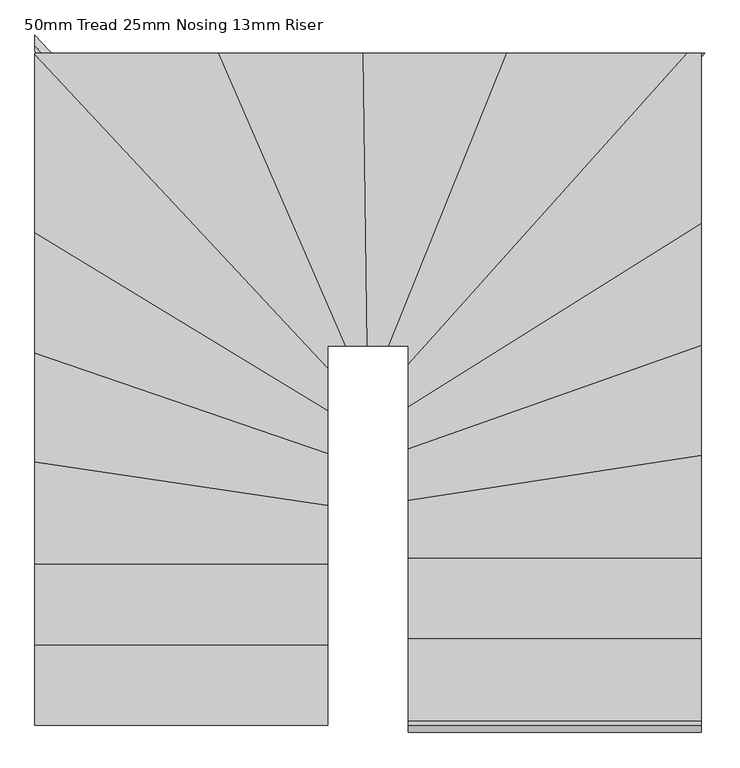
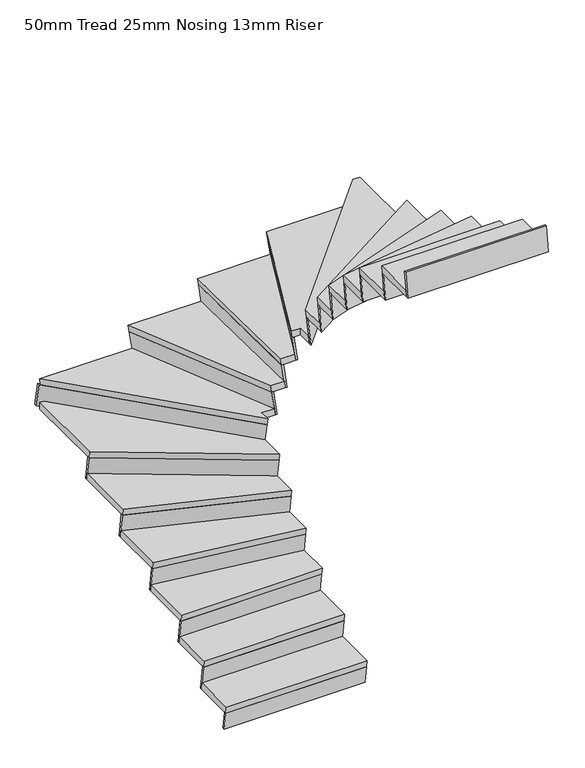
"""IFC4 building model written with IfcOpenShell, lengths in millimetres: stair flight geometry, 50mm Tread 25mm Nosing 13mm Riser."""

from ifc_helpers import new_model, si_unit, origin, place, context, project, spatial, faceted_brep, source, transform, mapped, element, save


def stair_flight_50mm_tread_25mm_nosing_13mm_riser_190ae62b(model_context):
    return source(origin(), model_context, "Body", "Brep", [
        faceted_brep([(10289.7497541, -1105.5848061, 179.2941176), (10289.7497541, -1098.6130213, 129.2941176), (9289.7239729, -1098.6130213, 129.2941176), (9289.7239729, -1105.5848061, 179.2941176), (9289.7239729, -1405.5848061, 179.2941176), (10289.7497541, -1405.5848061, 179.2941176), (10289.7497541, -1398.6130213, 129.2941176), (9289.7239729, -1398.6130213, 129.2941176)], [[[0, 1, 2, 3]], [[3, 4, 5, 0]], [[2, 1, 6, 7]], [[4, 3, 2, 7]], [[0, 5, 6, 1]], [[5, 4, 7, 6]]]),
        faceted_brep([(10289.7497541, -1398.6130213, 129.2941176), (10289.7497541, -1380.5848061, 0.0), (10289.7497541, -1367.9638766, 0.0), (10289.7497541, -1385.9920918, 129.2941176), (9289.7239729, -1398.6130213, 129.2941176), (9289.7239729, -1385.9920918, 129.2941176), (9289.7239729, -1367.9638766, 0.0), (9289.7239729, -1380.5848061, 0.0)], [[[0, 1, 2, 3]], [[4, 5, 6, 7]], [[1, 0, 4, 7]], [[2, 1, 7, 6]], [[3, 2, 6, 5]], [[0, 3, 5, 4]]]),
        faceted_brep([(10289.7497541, -1123.6130213, 308.5882353), (10289.7497541, -1098.6130213, 129.2941176), (10289.7497541, -1085.9920918, 129.2941176), (10289.7497541, -1110.9920918, 308.5882353), (9289.7239729, -1123.6130213, 308.5882353), (9289.7239729, -1110.9920918, 308.5882353), (9289.7239729, -1085.9920918, 129.2941176), (9289.7239729, -1098.6130213, 129.2941176)], [[[0, 1, 2, 3]], [[4, 5, 6, 7]], [[1, 0, 4, 7]], [[2, 1, 7, 6]], [[3, 2, 6, 5]], [[0, 3, 5, 4]]]),
        faceted_brep([(9289.7239729, -830.5848061, 358.5882353), (9289.7239729, -1130.5848061, 358.5882353), (10289.7497541, -1130.5848061, 358.5882353), (10289.7497541, -830.5848061, 358.5882353), (9289.7239729, -823.6130213, 308.5882353), (10289.7497541, -823.6130213, 308.5882353), (10289.7497541, -1123.6130213, 308.5882353), (9289.7239729, -1123.6130213, 308.5882353)], [[[0, 1, 2, 3]], [[4, 5, 6, 7]], [[1, 0, 4, 7]], [[3, 2, 6, 5]], [[3, 5, 4, 0]], [[2, 1, 7, 6]]]),
        faceted_brep([(10289.7497541, -848.6130213, 487.8823529), (10289.7497541, -823.6130213, 308.5882353), (10289.7497541, -810.9920918, 308.5882353), (10289.7497541, -835.9920918, 487.8823529), (9289.7239729, -848.6130213, 487.8823529), (9289.7239729, -835.9920918, 487.8823529), (9289.7239729, -810.9920918, 308.5882353), (9289.7239729, -823.6130213, 308.5882353)], [[[0, 1, 2, 3]], [[4, 5, 6, 7]], [[1, 0, 4, 7]], [[2, 1, 7, 6]], [[3, 2, 6, 5]], [[0, 3, 5, 4]]]),
        faceted_brep([(9289.7239729, -480.7581684, 537.8823529), (9289.7239729, -855.5848061, 537.8823529), (10289.7497541, -855.5848061, 537.8823529), (10289.7497541, -629.8587526, 537.8823529), (9289.7239729, -473.7093187, 487.8823529), (10289.7497541, -622.8099029, 487.8823529), (10289.7497541, -848.6130213, 487.8823529), (9289.7239729, -848.6130213, 487.8823529)], [[[0, 1, 2, 3]], [[4, 5, 6, 7]], [[1, 0, 4, 7]], [[3, 2, 6, 5]], [[3, 5, 4, 0]], [[2, 1, 7, 6]]]),
        faceted_brep([(10289.7497541, -648.0862485, 667.1764706), (10289.7497541, -622.8099029, 487.8823529), (10289.7497541, -610.0494638, 487.8823529), (10289.7497541, -635.3258095, 667.1764706), (9289.7239729, -498.9856643, 667.1764706), (9289.7239729, -486.2252253, 667.1764706), (9289.7239729, -460.9488796, 487.8823529), (9289.7239729, -473.7093187, 487.8823529)], [[[0, 1, 2, 3]], [[4, 5, 6, 7]], [[1, 0, 4, 7]], [[2, 1, 7, 6]], [[3, 2, 6, 5]], [[0, 3, 5, 4]]]),
        faceted_brep([(9289.7239729, -107.774321, 717.1764706), (9289.7239729, -506.034514, 717.1764706), (10289.7497541, -655.1350982, 717.1764706), (10289.7497541, -450.5397782, 717.1764706), (9289.7239729, -100.4043758, 667.1764706), (10289.7497541, -443.169833, 667.1764706), (10289.7497541, -648.0862485, 667.1764706), (9289.7239729, -498.9856643, 667.1764706)], [[[0, 1, 2, 3]], [[4, 5, 6, 7]], [[1, 0, 4, 7]], [[3, 2, 6, 5]], [[3, 5, 4, 0]], [[2, 1, 7, 6]]]),
        faceted_brep([(10289.7497541, -469.5975895, 846.4705882), (10289.7497541, -443.169833, 667.1764706), (10289.7497541, -429.8281189, 667.1764706), (10289.7497541, -456.2558754, 846.4705882), (9289.7239729, -126.8321323, 846.4705882), (9289.7239729, -113.4904182, 846.4705882), (9289.7239729, -87.0626618, 667.1764706), (9289.7239729, -100.4043758, 667.1764706)], [[[0, 1, 2, 3]], [[4, 5, 6, 7]], [[1, 0, 4, 7]], [[2, 1, 7, 6]], [[3, 2, 6, 5]], [[0, 3, 5, 4]]]),
        faceted_brep([(9289.7239729, 306.1026023, 896.4705882), (9289.7239729, -134.2020775, 896.4705882), (10289.7497541, -476.9675347, 896.4705882), (10289.7497541, -301.16869, 896.4705882), (9289.7239729, 314.2591716, 846.4705882), (10289.7497541, -293.0121207, 846.4705882), (10289.7497541, -469.5975895, 846.4705882), (9289.7239729, -126.8321323, 846.4705882)], [[[0, 1, 2, 3]], [[4, 5, 6, 7]], [[1, 0, 4, 7]], [[3, 2, 6, 5]], [[3, 5, 4, 0]], [[2, 1, 7, 6]]]),
        faceted_brep([(10289.7497541, -322.2606186, 1025.7647059), (10289.7497541, -293.0121207, 846.4705882), (10289.7497541, -278.2463915, 846.4705882), (10289.7497541, -307.4948894, 1025.7647059), (9289.7239729, 285.0106737, 1025.7647059), (9289.7239729, 299.7764029, 1025.7647059), (9289.7239729, 329.0249008, 846.4705882), (9289.7239729, 314.2591716, 846.4705882)], [[[0, 1, 2, 3]], [[4, 5, 6, 7]], [[1, 0, 4, 7]], [[2, 1, 7, 6]], [[3, 2, 6, 5]], [[0, 3, 5, 4]]]),
        faceted_brep([(9320.7227269, 889.7143644, 1075.7647059), (9289.7239729, 889.7143644, 1075.7647059), (9289.7239729, 276.8541044, 1075.7647059), (10289.7497541, -330.4171879, 1075.7647059), (10289.7497541, -148.9817857, 1075.7647059), (9330.2573955, 889.7143644, 1025.7647059), (10289.7497541, -138.761613, 1025.7647059), (10289.7497541, -322.2606186, 1025.7647059), (9289.7239729, 285.0106737, 1025.7647059), (9289.7239729, 889.7143644, 1025.7647059)], [[[0, 1, 2, 3, 4]], [[5, 6, 7, 8, 9]], [[1, 0, 5, 9]], [[4, 3, 7, 6]], [[4, 6, 5, 0]], [[3, 2, 8, 7]], [[2, 1, 9, 8]]]),
        faceted_brep([(10289.7497541, -175.4099498, 1205.0588235), (10289.7497541, -138.761613, 1025.7647059), (10289.7497541, -120.2601701, 1025.7647059), (10289.7497541, -156.9085068, 1205.0588235), (9289.7239729, 896.5136394, 1205.0588235), (9289.7239729, 915.0150824, 1205.0588235), (9289.7239729, 951.6634191, 1025.7647059), (9289.7239729, 933.1619761, 1025.7647059)], [[[0, 1, 2, 3]], [[4, 5, 6, 7]], [[1, 0, 4, 7]], [[2, 1, 7, 6]], [[3, 2, 6, 5]], [[0, 3, 5, 4]]]),
        faceted_brep([(9944.3142793, 889.7143644, 1255.0588235), (9289.7239729, 889.7143644, 1255.0588235), (9289.7239729, 886.2934667, 1255.0588235), (10289.7497541, -185.6301224, 1255.0588235), (10289.7497541, -110.3114169, 1255.0588235), (10378.5813525, -110.3114169, 1255.0588235), (9951.9150537, 889.7143644, 1205.0588235), (10386.182127, -110.3114169, 1205.0588235), (10289.7497541, -110.3114169, 1205.0588235), (10289.7497541, -175.4099498, 1205.0588235), (9296.0671958, 889.7143644, 1205.0588235), (9289.7239729, 889.7143644, 1238.3228165)], [[[0, 1, 2, 3, 4, 5]], [[6, 7, 8, 9, 10]], [[1, 0, 6, 10, 11]], [[2, 1, 11]], [[4, 3, 9, 8]], [[5, 4, 8, 7]], [[5, 7, 6, 0]], [[3, 2, 11, 10, 9]]]),
        faceted_brep([(10358.9266439, -110.3114169, 1384.3529412), (10386.182127, -110.3114169, 1205.0588235), (10399.9417081, -110.3114169, 1205.0588235), (10372.6862251, -110.3114169, 1384.3529412), (9924.6595707, 889.7143644, 1384.3529412), (9938.4191519, 889.7143644, 1384.3529412), (9965.6746349, 889.7143644, 1205.0588235), (9951.9150537, 889.7143644, 1205.0588235)], [[[0, 1, 2, 3]], [[4, 5, 6, 7]], [[1, 0, 4, 7]], [[2, 1, 7, 6]], [[3, 2, 6, 5]], [[0, 3, 5, 4]]]),
        faceted_brep([(10435.8300538, 889.7143644, 1434.3529412), (9917.0587962, 889.7143644, 1434.3529412), (10351.3258695, -110.3114169, 1434.3529412), (10449.7733926, -110.3114169, 1434.3529412), (10442.8025162, 889.7143644, 1384.3529412), (10456.745855, -110.3114169, 1384.3529412), (10358.9266439, -110.3114169, 1384.3529412), (9924.6595707, 889.7143644, 1384.3529412)], [[[0, 1, 2, 3]], [[4, 5, 6, 7]], [[1, 0, 4, 7]], [[3, 2, 6, 5]], [[3, 5, 4, 0]], [[2, 1, 7, 6]]]),
        faceted_brep([(10431.7434251, -110.3114169, 1563.6470588), (10456.745855, -110.3114169, 1384.3529412), (10469.3680113, -110.3114169, 1384.3529412), (10444.3655813, -110.3114169, 1563.6470588), (10417.8000863, 889.7143644, 1563.6470588), (10430.4222425, 889.7143644, 1563.6470588), (10455.4246725, 889.7143644, 1384.3529412), (10442.8025162, 889.7143644, 1384.3529412)], [[[0, 1, 2, 3]], [[4, 5, 6, 7]], [[1, 0, 4, 7]], [[2, 1, 7, 6]], [[3, 2, 6, 5]], [[0, 3, 5, 4]]]),
        faceted_brep([(10928.1794575, 889.7143644, 1613.6470588), (10410.8276238, 889.7143644, 1613.6470588), (10424.7709627, -110.3114169, 1613.6470588), (10523.7381228, -110.3114169, 1613.6470588), (10935.699827, 889.7143644, 1563.6470588), (10531.2584922, -110.3114169, 1563.6470588), (10431.7434251, -110.3114169, 1563.6470588), (10417.8000863, 889.7143644, 1563.6470588)], [[[0, 1, 2, 3]], [[4, 5, 6, 7]], [[1, 0, 4, 7]], [[3, 2, 6, 5]], [[3, 5, 4, 0]], [[2, 1, 7, 6]]]),
        faceted_brep([(10504.2913321, -110.3114169, 1742.9411765), (10531.2584922, -110.3114169, 1563.6470588), (10544.8725173, -110.3114169, 1563.6470588), (10517.9053572, -110.3114169, 1742.9411765), (10908.7326669, 889.7143644, 1742.9411765), (10922.346692, 889.7143644, 1742.9411765), (10949.3138521, 889.7143644, 1563.6470588), (10935.699827, 889.7143644, 1563.6470588)], [[[0, 1, 2, 3]], [[4, 5, 6, 7]], [[1, 0, 4, 7]], [[2, 1, 7, 6]], [[3, 2, 6, 5]], [[0, 3, 5, 4]]]),
        faceted_brep([(11550.6912543, 889.7143644, 1792.9411765), (10901.2122974, 889.7143644, 1792.9411765), (10496.7709627, -110.3114169, 1792.9411765), (10564.7497541, -110.3114169, 1792.9411765), (10564.7497541, -211.248652, 1792.9411765), (11560.0499961, 889.7143644, 1742.9411765), (10564.7497541, -221.6991996, 1742.9411765), (10564.7497541, -110.3114169, 1742.9411765), (10504.2913321, -110.3114169, 1742.9411765), (10908.7326669, 889.7143644, 1742.9411765)], [[[0, 1, 2, 3, 4]], [[5, 6, 7, 8, 9]], [[1, 0, 5, 9]], [[3, 2, 8, 7]], [[4, 3, 7, 6]], [[4, 6, 5, 0]], [[2, 1, 9, 8]]]),
        faceted_brep([(10564.7497541, -184.2247655, 1922.2352941), (10564.7497541, -221.6991996, 1742.9411765), (10564.7497541, -240.6176872, 1742.9411765), (10564.7497541, -203.1432531, 1922.2352941), (11526.4906492, 889.7143644, 1922.2352941), (11543.4326552, 889.7143644, 1922.2352941), (11576.9920021, 889.7143644, 1742.9411765), (11560.0499961, 889.7143644, 1742.9411765)], [[[0, 1, 2, 3]], [[4, 5, 6, 7]], [[1, 0, 4, 7]], [[2, 1, 7, 6]], [[3, 2, 6, 5]], [[0, 3, 5, 4]]]),
        faceted_brep([(11564.7755354, 278.4528718, 1972.2352941), (11564.7755354, 889.7143644, 1972.2352941), (11517.1319075, 889.7143644, 1972.2352941), (10564.7497541, -173.7742179, 1972.2352941), (10564.7497541, -348.5530054, 1972.2352941), (11564.7755354, 270.2240506, 1922.2352941), (10564.7497541, -356.7818266, 1922.2352941), (10564.7497541, -184.2247655, 1922.2352941), (11526.4906492, 889.7143644, 1922.2352941), (11564.7755354, 889.7143644, 1922.2352941)], [[[0, 1, 2, 3, 4]], [[5, 6, 7, 8, 9]], [[1, 0, 5, 9]], [[2, 1, 9, 8]], [[4, 3, 7, 6]], [[4, 6, 5, 0]], [[3, 2, 8, 7]]]),
        faceted_brep([(10564.7497541, -327.2742418, 2101.5294118), (10564.7497541, -356.7818266, 1922.2352941), (10564.7497541, -371.6783525, 1922.2352941), (10564.7497541, -342.1707677, 2101.5294118), (11564.7755354, 299.7316354, 2101.5294118), (11564.7755354, 284.8351095, 2101.5294118), (11564.7755354, 255.3275247, 1922.2352941), (11564.7755354, 270.2240506, 1922.2352941)], [[[0, 1, 2, 3]], [[4, 5, 6, 7]], [[1, 0, 4, 7]], [[2, 1, 7, 6]], [[3, 2, 6, 5]], [[0, 3, 5, 4]]]),
        faceted_brep([(11564.7755354, -136.4321631, 2151.5294118), (11564.7755354, 307.9604567, 2151.5294118), (10564.7497541, -319.0454205, 2151.5294118), (10564.7497541, -489.6437867, 2151.5294118), (11564.7755354, -143.8260425, 2101.5294118), (10564.7497541, -497.0376661, 2101.5294118), (10564.7497541, -327.2742418, 2101.5294118), (11564.7755354, 299.7316354, 2101.5294118)], [[[0, 1, 2, 3]], [[4, 5, 6, 7]], [[1, 0, 4, 7]], [[3, 2, 6, 5]], [[3, 5, 4, 0]], [[2, 1, 7, 6]]]),
        faceted_brep([(10564.7497541, -470.5240844, 2280.8235294), (10564.7497541, -497.0376661, 2101.5294118), (10564.7497541, -510.4227078, 2101.5294118), (10564.7497541, -483.9091262, 2280.8235294), (11564.7755354, -117.3124608, 2280.8235294), (11564.7755354, -130.6975026, 2280.8235294), (11564.7755354, -157.2110842, 2101.5294118), (11564.7755354, -143.8260425, 2101.5294118)], [[[0, 1, 2, 3]], [[4, 5, 6, 7]], [[1, 0, 4, 7]], [[2, 1, 7, 6]], [[3, 2, 6, 5]], [[0, 3, 5, 4]]]),
        faceted_brep([(11564.7755354, -509.957846, 2330.8235294), (11564.7755354, -109.9185814, 2330.8235294), (10564.7497541, -463.130205, 2330.8235294), (10564.7497541, -663.6782099, 2330.8235294), (11564.7755354, -517.0115171, 2280.8235294), (10564.7497541, -670.731881, 2280.8235294), (10564.7497541, -470.5240844, 2280.8235294), (11564.7755354, -117.3124608, 2280.8235294)], [[[0, 1, 2, 3]], [[4, 5, 6, 7]], [[1, 0, 4, 7]], [[3, 2, 6, 5]], [[3, 5, 4, 0]], [[2, 1, 7, 6]]]),
        faceted_brep([(10564.7497541, -645.4382463, 2460.1176471), (10564.7497541, -670.731881, 2280.8235294), (10564.7497541, -683.5010482, 2280.8235294), (10564.7497541, -658.2074135, 2460.1176471), (11564.7755354, -491.7178824, 2460.1176471), (11564.7755354, -504.4870496, 2460.1176471), (11564.7755354, -529.7806843, 2280.8235294), (11564.7755354, -517.0115171, 2280.8235294)], [[[0, 1, 2, 3]], [[4, 5, 6, 7]], [[1, 0, 4, 7]], [[2, 1, 7, 6]], [[3, 2, 6, 5]], [[0, 3, 5, 4]]]),
        faceted_brep([(11564.7755354, -861.5243932, 2510.1176471), (11564.7755354, -484.6642113, 2510.1176471), (10564.7497541, -638.3845752, 2510.1176471), (10564.7497541, -861.5243932, 2510.1176471), (11564.7755354, -868.496178, 2460.1176471), (10564.7497541, -868.496178, 2460.1176471), (10564.7497541, -645.4382463, 2460.1176471), (11564.7755354, -491.7178824, 2460.1176471)], [[[0, 1, 2, 3]], [[4, 5, 6, 7]], [[1, 0, 4, 7]], [[3, 2, 6, 5]], [[3, 5, 4, 0]], [[2, 1, 7, 6]]]),
        faceted_brep([(10564.7497541, -843.496178, 2639.4117647), (10564.7497541, -868.496178, 2460.1176471), (10564.7497541, -881.1171075, 2460.1176471), (10564.7497541, -856.1171075, 2639.4117647), (11564.7755354, -843.496178, 2639.4117647), (11564.7755354, -856.1171075, 2639.4117647), (11564.7755354, -881.1171075, 2460.1176471), (11564.7755354, -868.496178, 2460.1176471)], [[[0, 1, 2, 3]], [[4, 5, 6, 7]], [[1, 0, 4, 7]], [[2, 1, 7, 6]], [[3, 2, 6, 5]], [[0, 3, 5, 4]]]),
        faceted_brep([(11564.7755354, -1136.5243932, 2689.4117647), (11564.7755354, -836.5243932, 2689.4117647), (10564.7497541, -836.5243932, 2689.4117647), (10564.7497541, -1136.5243932, 2689.4117647), (11564.7755354, -1143.496178, 2639.4117647), (10564.7497541, -1143.496178, 2639.4117647), (10564.7497541, -843.496178, 2639.4117647), (11564.7755354, -843.496178, 2639.4117647)], [[[0, 1, 2, 3]], [[4, 5, 6, 7]], [[1, 0, 4, 7]], [[3, 2, 6, 5]], [[3, 5, 4, 0]], [[2, 1, 7, 6]]]),
        faceted_brep([(10564.7497541, -1118.496178, 2818.7058824), (10564.7497541, -1143.496178, 2639.4117647), (10564.7497541, -1156.1171075, 2639.4117647), (10564.7497541, -1131.1171075, 2818.7058824), (11564.7755354, -1118.496178, 2818.7058824), (11564.7755354, -1131.1171075, 2818.7058824), (11564.7755354, -1156.1171075, 2639.4117647), (11564.7755354, -1143.496178, 2639.4117647)], [[[0, 1, 2, 3]], [[4, 5, 6, 7]], [[1, 0, 4, 7]], [[2, 1, 7, 6]], [[3, 2, 6, 5]], [[0, 3, 5, 4]]]),
        faceted_brep([(10564.7497541, -1393.496178, 2998.0), (10564.7497541, -1418.496178, 2818.7058824), (10564.7497541, -1431.1171075, 2818.7058824), (10564.7497541, -1406.1171075, 2998.0), (11564.7755354, -1393.496178, 2998.0), (11564.7755354, -1406.1171075, 2998.0), (11564.7755354, -1431.1171075, 2818.7058824), (11564.7755354, -1418.496178, 2818.7058824)], [[[0, 1, 2, 3]], [[4, 5, 6, 7]], [[1, 0, 4, 7]], [[2, 1, 7, 6]], [[3, 2, 6, 5]], [[0, 3, 5, 4]]]),
        faceted_brep([(11564.7755354, -1411.5243932, 2868.7058824), (11564.7755354, -1111.5243932, 2868.7058824), (10564.7497541, -1111.5243932, 2868.7058824), (10564.7497541, -1411.5243932, 2868.7058824), (11564.7755354, -1418.496178, 2818.7058824), (10564.7497541, -1418.496178, 2818.7058824), (10564.7497541, -1118.496178, 2818.7058824), (11564.7755354, -1118.496178, 2818.7058824)], [[[0, 1, 2, 3]], [[4, 5, 6, 7]], [[1, 0, 4, 7]], [[3, 2, 6, 5]], [[3, 5, 4, 0]], [[2, 1, 7, 6]]]),
    ])


if __name__ == "__main__":
    model = new_model("IFC4")
    model_context = context("Model", 3, world=origin())
    ifc_project = project(units=[si_unit("LENGTHUNIT", "METRE", prefix="MILLI")], contexts=[model_context])
    site = spatial("IfcSite", under=ifc_project)
    building = spatial("IfcBuilding", under=site)
    placement = place(None, origin())
    stair_flight_50mm_tread_25mm_nosing_13mm_riser_shape = stair_flight_50mm_tread_25mm_nosing_13mm_riser_190ae62b(model_context)
    element("IfcStairFlight", 1, ObjectType="50mm Tread 25mm Nosing 13mm Riser", at=placement, inside=building, context=model_context, shape_type="MappedRepresentation", body=[
        mapped(stair_flight_50mm_tread_25mm_nosing_13mm_riser_shape, transform((0.0, 0.0, 0.0), x_axis=(1.0, 0.0, 0.0), y_axis=(0.0, 1.0, 0.0), z_axis=(0.0, 0.0, 1.0))),
    ])
    save(model, "model.ifc")
